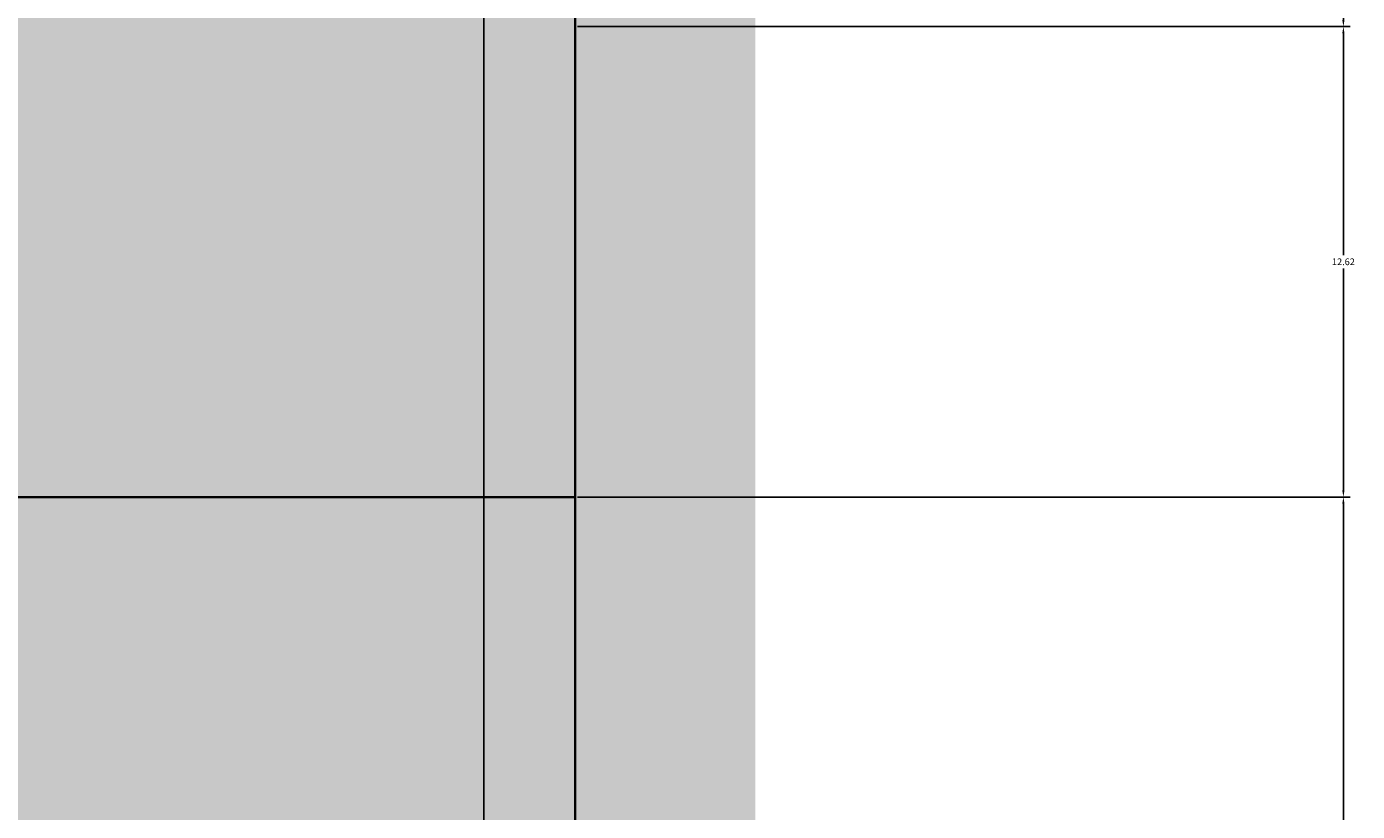
# Model space of a CAD drawing. Units: feet. Extents: x 2695 to 2912, y 795 to 1139.
# Tile 78 of 83: x 2876 to 2912, y 1042 to 1063. Entities that reach past the tile are written whole.
import ezdxf

# ---------------------------------------------------------------- set-up
doc = ezdxf.new("R2010")
doc.units = ezdxf.units.FT
for name, color, linetype, lineweight in [('A-ANNO-DIMS', 2, 'Continuous', 18), ('A-ELEV', 7, 'Continuous', 35), ('A-ELEV-PATT', 252, 'Continuous', 13)]:
    doc.layers.add(name, color=color, linetype=linetype, lineweight=lineweight)
doc.styles.get("Standard").update_dxf_attribs({"font": 'arial.ttf'})
doc.dimstyles.get("Standard").update_dxf_attribs({"dimtxt": 0.18, "dimasz": 0.18, "dimexe": 0.18, "dimexo": 0.0625, "dimgap": 0.09, "dimtad": 0, "dimtih": 1, "dimtoh": 1, "dimdec": 1, "dimzin": 0, "dimdsep": 46, "dimlunit": 3, "dimtxsty": 'Standard', "dimcen": 0.09, "dimadec": 0, "dimazin": 0, "dimtfac": 1, "dimtdec": 1, "dimtofl": 0, "dimtmove": 0, "dimatfit": 3, "dimfxl": 1, "dimtolj": 1, "dimtzin": 0, "dimarcsym": 0})

# ---------------------------------------------------------------- blocks, each defined once
blk = doc.blocks.new('*D11')
at = {"layer": 'A-ANNO-DIMS', "color": 0, "lineweight": -2, "transparency": 16777216}
for p, q in [((2843.575, 1020.886), (2843.575, 1138.886)), ((2843.755, 1138.706), (2869.128, 1138.706)), ((2895.289, 1138.706), (2869.916, 1138.706)), ((2895.469, 1107.898), (2895.469, 1138.886))]:
    blk.add_line(p, q, dxfattribs=at)
at = {"layer": 'A-ANNO-DIMS', "color": 0, "transparency": 16777216}
for points in [[(2843.755, 1138.736), (2843.755, 1138.676), (2843.575, 1138.706)], [(2895.289, 1138.736), (2895.289, 1138.676), (2895.469, 1138.706)]]:
    blk.add_solid(points, dxfattribs=at)
at = {"layer": 'Defpoints', "color": 0, "transparency": 16777216}
for p in [(2895.469, 1138.706), (2895.469, 1107.835), (2843.575, 1020.824)]:
    blk.add_point(p, dxfattribs=at)
at = {"layer": 'A-ANNO-DIMS', "color": 0, "transparency": 16777216, "insert": (2869.522, 1138.706), "char_height": 0.18, "attachment_point": 5}
blk.add_mtext('\\A1;51.89', dxfattribs=at)
blk = doc.blocks.new('*D18')
at = {"layer": 'A-ANNO-DIMS', "color": 0, "lineweight": -2, "transparency": 16777216}
for p, q in [((2890.699, 1050.311), (2911.424, 1050.311)), ((2911.244, 1050.131), (2911.244, 1035.749)), ((2911.244, 1021.004), (2911.244, 1035.385)), ((2843.637, 1020.824), (2911.424, 1020.824))]:
    blk.add_line(p, q, dxfattribs=at)
at = {"layer": 'A-ANNO-DIMS', "color": 0, "transparency": 16777216}
for points in [[(2911.214, 1050.131), (2911.274, 1050.131), (2911.244, 1050.311)], [(2911.214, 1021.004), (2911.274, 1021.004), (2911.244, 1020.824)]]:
    blk.add_solid(points, dxfattribs=at)
at = {"layer": 'Defpoints', "color": 0, "transparency": 16777216}
for p in [(2890.636, 1050.311), (2911.244, 1050.311), (2843.575, 1020.824)]:
    blk.add_point(p, dxfattribs=at)
at = {"layer": 'A-ANNO-DIMS', "color": 0, "transparency": 16777216, "insert": (2911.244, 1035.567), "char_height": 0.18, "attachment_point": 5}
blk.add_mtext('\\A1;29.487', dxfattribs=at)
blk = doc.blocks.new('*D19')
at = {"layer": 'A-ANNO-DIMS', "color": 0, "lineweight": -2, "transparency": 16777216}
for p, q in [((2890.699, 1062.931), (2911.424, 1062.931)), ((2911.244, 1062.751), (2911.244, 1056.802)), ((2911.244, 1050.491), (2911.244, 1056.439)), ((2890.699, 1050.311), (2911.424, 1050.311))]:
    blk.add_line(p, q, dxfattribs=at)
at = {"layer": 'A-ANNO-DIMS', "color": 0, "transparency": 16777216}
for points in [[(2911.214, 1062.751), (2911.274, 1062.751), (2911.244, 1062.931)], [(2911.214, 1050.491), (2911.274, 1050.491), (2911.244, 1050.311)]]:
    blk.add_solid(points, dxfattribs=at)
at = {"layer": 'Defpoints', "color": 0, "transparency": 16777216}
for p in [(2890.636, 1062.931), (2911.244, 1062.931), (2890.636, 1050.311)]:
    blk.add_point(p, dxfattribs=at)
at = {"layer": 'A-ANNO-DIMS', "color": 0, "transparency": 16777216, "insert": (2911.244, 1056.621), "char_height": 0.18, "attachment_point": 5}
blk.add_mtext('\\A1;12.62', dxfattribs=at)
blk = doc.blocks.new('*D20')
at = {"layer": 'A-ANNO-DIMS', "color": 0, "lineweight": -2, "transparency": 16777216}
for p, q in [((2895.532, 1103.338), (2911.424, 1103.338)), ((2911.244, 1103.158), (2911.244, 1083.316)), ((2911.244, 1063.111), (2911.244, 1082.952)), ((2890.699, 1062.931), (2911.424, 1062.931))]:
    blk.add_line(p, q, dxfattribs=at)
at = {"layer": 'A-ANNO-DIMS', "color": 0, "transparency": 16777216}
for points in [[(2911.214, 1103.158), (2911.274, 1103.158), (2911.244, 1103.338)], [(2911.214, 1063.111), (2911.274, 1063.111), (2911.244, 1062.931)]]:
    blk.add_solid(points, dxfattribs=at)
at = {"layer": 'Defpoints', "color": 0, "transparency": 16777216}
for p in [(2895.469, 1103.338), (2911.244, 1103.338), (2890.636, 1062.931)]:
    blk.add_point(p, dxfattribs=at)
at = {"layer": 'A-ANNO-DIMS', "color": 0, "transparency": 16777216, "insert": (2911.244, 1083.134), "char_height": 0.18, "attachment_point": 5}
blk.add_mtext('\\A1;40.41', dxfattribs=at)
blk = doc.blocks.new('*D50')
at = {"layer": 'A-ANNO-DIMS', "color": 0, "lineweight": -2, "transparency": 16777216}
for p, q in [((2810.041, 972.03), (2810.041, 1138.886)), ((2810.221, 1138.706), (2848.721, 1138.706)), ((2888.008, 1138.706), (2849.508, 1138.706)), ((2888.188, 972.03), (2888.188, 1138.886))]:
    blk.add_line(p, q, dxfattribs=at)
at = {"layer": 'A-ANNO-DIMS', "color": 0, "transparency": 16777216}
for points in [[(2810.221, 1138.736), (2810.221, 1138.676), (2810.041, 1138.706)], [(2888.008, 1138.736), (2888.008, 1138.676), (2888.188, 1138.706)]]:
    blk.add_solid(points, dxfattribs=at)
at = {"layer": 'Defpoints', "color": 0, "transparency": 16777216}
for p in [(2888.188, 1138.706), (2810.041, 971.967), (2888.188, 971.967)]:
    blk.add_point(p, dxfattribs=at)
at = {"layer": 'A-ANNO-DIMS', "color": 0, "transparency": 16777216, "insert": (2849.114, 1138.706), "char_height": 0.18, "attachment_point": 5}
blk.add_mtext('\\A1;78.15', dxfattribs=at)
blk = doc.blocks.new('*D51')
at = {"layer": 'A-ANNO-DIMS', "color": 0, "lineweight": -2, "transparency": 16777216}
for p, q in [((2888.188, 972.03), (2888.188, 1138.886)), ((2888.368, 1138.706), (2889.017, 1138.706)), ((2890.456, 1138.706), (2889.808, 1138.706)), ((2890.636, 972.03), (2890.636, 1138.886))]:
    blk.add_line(p, q, dxfattribs=at)
at = {"layer": 'A-ANNO-DIMS', "color": 0, "transparency": 16777216}
for points in [[(2888.368, 1138.736), (2888.368, 1138.676), (2888.188, 1138.706)], [(2890.456, 1138.736), (2890.456, 1138.676), (2890.636, 1138.706)]]:
    blk.add_solid(points, dxfattribs=at)
at = {"layer": 'Defpoints', "color": 0, "transparency": 16777216}
for p in [(2890.636, 1138.706), (2888.188, 971.967), (2890.636, 971.967)]:
    blk.add_point(p, dxfattribs=at)
at = {"layer": 'A-ANNO-DIMS', "color": 0, "transparency": 16777216, "insert": (2889.412, 1138.706), "char_height": 0.18, "attachment_point": 5}
blk.add_mtext('\\A1;2.448', dxfattribs=at)

msp = doc.modelspace()

# ---------------------------------------------------------------- hatches: boundary and pattern name
at = {"layer": 'A-ELEV-PATT'}
h = msp.add_hatch(color=256, dxfattribs=at)
h.set_gradient(color1=(255, 255, 255), tint=1)
h.paths.add_polyline_path([(2770.6361, 1122.9306), (2710.6361, 1122.9306), (2710.6361, 1118.4096), (2770.6361, 1118.4096)])
h.paths.add_polyline_path([(2890.6361, 1107.8588), (2770.6361, 1107.8588), (2770.6361, 1103.3378), (2890.6361, 1103.3378)])
h.paths.add_polyline_path([(2890.6361, 1062.9306), (2710.6361, 1062.9306), (2710.6361, 1056.9306), (2710.6361, 936.9306), (2710.6361, 924.3105), (2716.5358, 924.3105), (2890.6361, 924.3105), (2890.6361, 936.9306), (2715.8852, 936.9306), (2715.8852, 1050.3105), (2890.6361, 1050.3105)])
h.paths.add_polyline_path([(2716.5358, 924.3105), (2710.6361, 924.3105), (2710.6361, 810.9306), (2716.5358, 810.9306)])
h = msp.add_hatch(color=256, dxfattribs=at)
h.set_gradient(color1=(147, 149, 152), color2=(147, 149, 152), tint=1)
h.paths.add_polyline_path([(2770.6361, 1118.4096), (2710.6361, 1118.4096), (2710.6361, 1062.9306), (2770.6361, 1062.9306)])
h.paths.add_polyline_path([(2890.6361, 1103.3378), (2770.6361, 1103.3378), (2770.6361, 1062.9306), (2890.6361, 1062.9306)])
h.paths.add_polyline_path([(2730.7081, 1048.1052), (2755.1125, 1048.1052), (2755.1125, 936.9306), (2770.6361, 936.9306), (2770.6361, 1050.3105), (2715.8852, 1050.3105), (2715.8852, 936.9306), (2730.7081, 936.9306)])
h.paths.add_polyline_path([(2890.6361, 1050.3105), (2770.6361, 1050.3105), (2770.6361, 971.9673), (2778.0341, 971.9673), (2778.0341, 1020.8235), (2843.575, 1020.8235), (2843.575, 971.9673), (2890.6361, 971.9673)])
h.paths.add_polyline_path([(2888.1882, 970.7156), (2843.575, 970.7156), (2843.575, 964.8267), (2888.1882, 964.8267)])
h.paths.add_polyline_path([(2888.1882, 964.1328), (2843.575, 964.1328), (2843.575, 956.614), (2888.1882, 956.614)])
h.paths.add_polyline_path([(2888.1882, 955.9202), (2843.575, 955.9202), (2843.575, 949.2892), (2888.1882, 949.2892)])
h.paths.add_polyline_path([(2888.1882, 948.5954), (2843.575, 948.5954), (2843.575, 941.3507), (2888.1882, 941.3507)])
h.paths.add_polyline_path([(2888.1882, 940.6569), (2843.575, 940.6569), (2843.575, 936.9306), (2888.1882, 936.9306)])
h.paths.add_polyline_path([(2890.6361, 970.7156), (2888.9368, 970.7156), (2888.9368, 964.8267), (2890.6361, 964.8267)])
h.paths.add_polyline_path([(2890.6361, 964.1328), (2888.9368, 964.1328), (2888.9368, 956.614), (2890.6361, 956.614)])
h.paths.add_polyline_path([(2890.6361, 955.9202), (2888.9368, 955.9202), (2888.9368, 949.2892), (2890.6361, 949.2892)])
h.paths.add_polyline_path([(2890.6361, 940.6569), (2888.9368, 940.6569), (2888.9368, 936.9306), (2890.6361, 936.9306)])
h.paths.add_polyline_path([(2890.6361, 948.5954), (2888.9368, 948.5954), (2888.9368, 941.3507), (2890.6361, 941.3507)])
h.paths.add_polyline_path([(2772.5216, 970.7156), (2770.6361, 970.7156), (2770.6361, 964.8267), (2772.5216, 964.8267)])
h.paths.add_polyline_path([(2772.5216, 964.1328), (2770.6361, 964.1328), (2770.6361, 956.614), (2772.5216, 956.614)])
h.paths.add_polyline_path([(2772.5216, 955.9202), (2770.6361, 955.9202), (2770.6361, 949.2892), (2772.5216, 949.2892)])
h.paths.add_polyline_path([(2772.5216, 948.5954), (2770.6361, 948.5954), (2770.6361, 941.3507), (2772.5216, 941.3507)])
h.paths.add_polyline_path([(2772.5216, 940.6569), (2770.6361, 940.6569), (2770.6361, 936.9306), (2772.5216, 936.9306)])
h.paths.add_polyline_path([(2778.0341, 940.6569), (2773.2702, 940.6569), (2773.2702, 936.9306), (2778.0341, 936.9306)])
h.paths.add_polyline_path([(2778.0341, 970.7156), (2773.2702, 970.7156), (2773.2702, 964.8267), (2778.0341, 964.8267)])
h.paths.add_polyline_path([(2778.0341, 964.1328), (2773.2702, 964.1328), (2773.2702, 956.614), (2778.0341, 956.614)])
h.paths.add_polyline_path([(2778.0341, 955.9202), (2773.2702, 955.9202), (2773.2702, 949.2892), (2778.0341, 949.2892)])
h.paths.add_polyline_path([(2778.0341, 948.5954), (2773.2702, 948.5954), (2773.2702, 941.3507), (2778.0341, 941.3507)])
h.paths.add_polyline_path([(2810.0407, 940.6569), (2780.0341, 940.6569), (2780.0341, 936.9306), (2810.0407, 936.9306)])
h.paths.add_polyline_path([(2890.6361, 924.3105), (2770.6361, 924.3105), (2770.6361, 810.9306), (2773.5029, 810.9306), (2773.5029, 905.5143), (2805.9398, 905.5143), (2838.3767, 905.5143), (2838.3767, 810.9306), (2890.6361, 810.9306)])
h = msp.add_hatch(color=256, dxfattribs=at)
h.set_gradient(color1=(255, 255, 255), tint=1)
h.paths.add_polyline_path([(2895.4694, 1107.8588), (2890.6361, 1107.8588), (2890.6361, 810.9306), (2895.4694, 810.9306)])
h = msp.add_hatch(color=256, dxfattribs=at)
h.set_gradient(color1=(255, 255, 255), tint=1)
h.paths.add_polyline_path([(2890.6361, 1050.3105), (2881.9484, 1050.3105), (2881.9484, 971.9673), (2890.6361, 971.9673)])
h.paths.add_polyline_path([(2888.1882, 970.7156), (2881.9484, 970.7156), (2881.9484, 964.8267), (2888.1882, 964.8267)])
h.paths.add_polyline_path([(2890.6361, 970.7156), (2888.9368, 970.7156), (2888.9368, 964.8267), (2890.6361, 964.8267)])
h.paths.add_polyline_path([(2888.1882, 964.1328), (2881.9484, 964.1328), (2881.9484, 956.614), (2888.1882, 956.614)])
h.paths.add_polyline_path([(2890.6361, 964.1328), (2888.9368, 964.1328), (2888.9368, 956.614), (2890.6361, 956.614)])
h.paths.add_polyline_path([(2888.1882, 955.9202), (2881.9484, 955.9202), (2881.9484, 949.2892), (2888.1882, 949.2892)])
h.paths.add_polyline_path([(2890.6361, 955.9202), (2888.9368, 955.9202), (2888.9368, 949.2892), (2890.6361, 949.2892)])
h.paths.add_polyline_path([(2888.1882, 948.5954), (2881.9484, 948.5954), (2881.9484, 941.3507), (2888.1882, 941.3507)])
h.paths.add_polyline_path([(2890.6361, 948.5954), (2888.9368, 948.5954), (2888.9368, 941.3507), (2890.6361, 941.3507)])
h.paths.add_polyline_path([(2888.1882, 940.6569), (2881.9484, 940.6569), (2881.9484, 936.9306), (2888.1882, 936.9306)])

# ---------------------------------------------------------------- linework, layer by layer
at = {"layer": 'A-ELEV'}
for p, q in [((2890.6361, 810.9306), (2890.6361, 1107.8588)), ((2890.6361, 1062.9306), (2890.6361, 810.9306)), ((2890.6361, 1050.3105), (2715.8852, 1050.3105))]:
    msp.add_line(p, q, dxfattribs=at)
msp.add_lwpolyline([(2890.6361, 1050.3105), (2715.8852, 1050.3105)], dxfattribs=at)

# ---------------------------------------------------------------- dimensions: what is measured, and where the dimension line sits
at = {"layer": 'A-ANNO-DIMS'}
for base, p1, p2, override, picture, middle in [((2888.1882, 1138.7056), (2810.0407, 971.9673), (2888.1882, 971.9673), {"dimdec": 2, "dimlfac": 1, "dimrnd": 0, "dimzin": 0, "dimdsep": 46, "dimlunit": 2}, '*D50', (2849.1144, 1138.7056)), ((2895.4694, 1138.7056), (2843.575, 1020.8235), (2895.4694, 1107.8352), {"dimdec": 2, "dimlfac": 1, "dimrnd": 0, "dimzin": 0, "dimdsep": 46, "dimlunit": 2}, '*D11', (2869.5222, 1138.7056)), ((2890.6361, 1138.7056), (2888.1882, 971.9673), (2890.6361, 971.9673), {"dimdec": 3, "dimlfac": 1, "dimrnd": 0, "dimzin": 0, "dimdsep": 46, "dimlunit": 2}, '*D51', (2889.4121, 1138.7056))]:
    dim = msp.add_linear_dim(base=base, p1=p1, p2=p2, dimstyle='Standard', override=override, dxfattribs=at)
    dim.commit()
    dim.dimension.update_dxf_attribs({"geometry": picture, "text_midpoint": middle})
for base, p1, p2, override, picture, middle in [((2911.2444, 1103.3378), (2890.6361, 1062.9306), (2895.4694, 1103.3378), {"dimdec": 2, "dimlfac": 1, "dimrnd": 0, "dimzin": 0, "dimdsep": 46, "dimlunit": 2}, '*D20', (2911.2444, 1083.1342)), ((2911.2444, 1062.9306), (2890.6361, 1050.3105), (2890.6361, 1062.9306), {"dimdec": 2, "dimlfac": 1, "dimrnd": 0, "dimzin": 0, "dimdsep": 46, "dimlunit": 2}, '*D19', (2911.2444, 1056.6206)), ((2911.2444, 1050.3105), (2843.575, 1020.8235), (2890.6361, 1050.3105), {"dimdec": 3, "dimlfac": 1, "dimrnd": 0, "dimzin": 0, "dimdsep": 46, "dimlunit": 2}, '*D18', (2911.2444, 1035.567))]:
    dim = msp.add_linear_dim(base=base, p1=p1, p2=p2, angle=90, dimstyle='Standard', override=override, dxfattribs=at)
    dim.commit()
    dim.dimension.update_dxf_attribs({"geometry": picture, "text_midpoint": middle})

doc.saveas('drawing.dxf')
